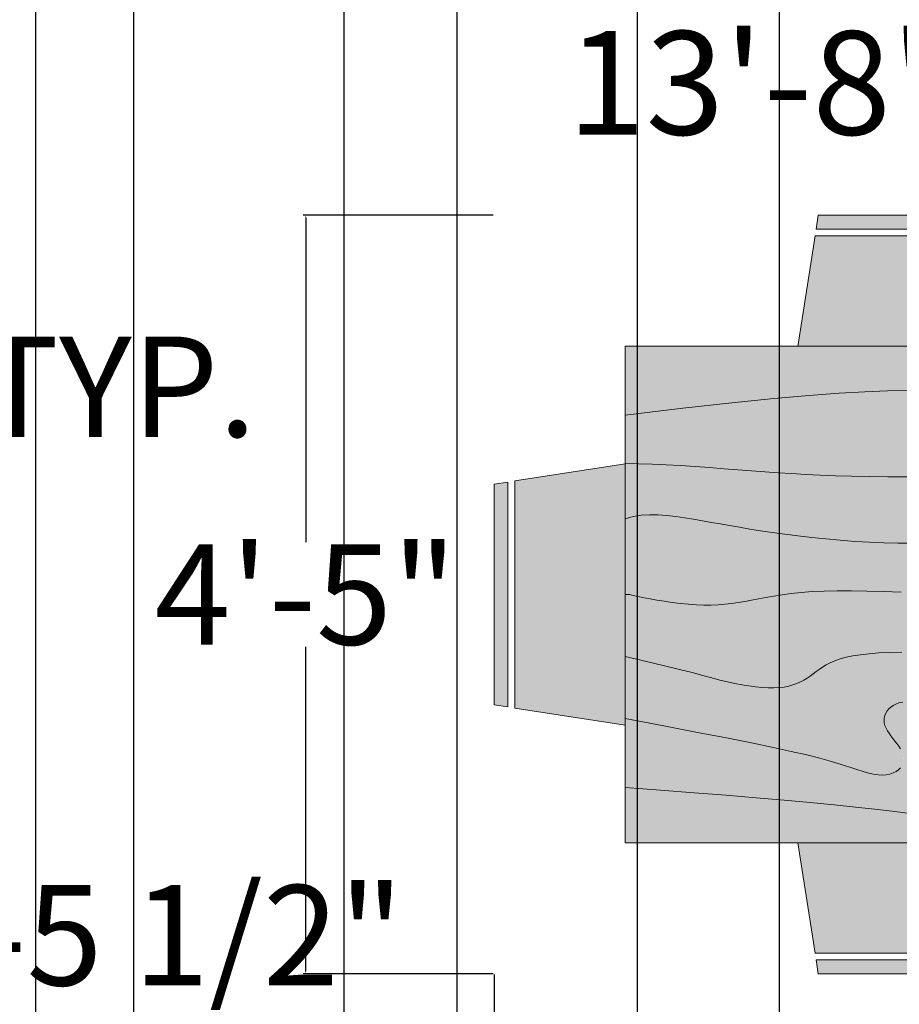
# Model space of a CAD drawing. Units: inches. Extents: x 2974 to 3443, y 2405 to 2963.
# Tile 5 of 13: x 3214 to 3276, y 2642 to 2711. Entities that reach past the tile are written whole.
import ezdxf

# ---------------------------------------------------------------- set-up
doc = ezdxf.new("R2010")
doc.units = ezdxf.units.IN
doc.header["$MEASUREMENT"] = 0
doc.layers.get('0').update_dxf_attribs({"color": 251})
for name, color, linetype, lineweight in [('A-ANNO-DIMS', 2, 'Continuous', 18), ('A-AREA-IDEN', 250, 'Continuous', 25), ('furniture', 32, 'Continuous', 18)]:
    doc.layers.add(name, color=color, linetype=linetype, lineweight=lineweight)
doc.layers.add('A-FURN-PATT', color=254, linetype='Continuous', lineweight=13, true_color=0xfeeab9)
doc.styles.get("Standard").update_dxf_attribs({"font": 'arial.ttf'})
doc.dimstyles.get("Standard").update_dxf_attribs({"dimtxt": 7, "dimasz": 0.18, "dimexe": 0.18, "dimexo": 0.0625, "dimgap": 0.09, "dimtad": 0, "dimtih": 1, "dimtoh": 1, "dimzin": 0, "dimdsep": 46, "dimlunit": 3, "dimtxsty": 'Standard', "dimcen": 0.09, "dimadec": 0, "dimazin": 0, "dimtfac": 1, "dimtofl": 0, "dimtmove": 0, "dimatfit": 3, "dimfxl": 1, "dimtolj": 1, "dimtzin": 0, "dimarcsym": 0})

# ---------------------------------------------------------------- blocks, each defined once
blk = doc.blocks.new('Dining Set - 36 x 72 in.')
for p, q in [((6, 27.5), (22, 27.5)), ((22.1563, 26.49966), (22, 27.5)), ((22.1584, 26.5), (5.8466, 26.5)), ((5.7696, 26), (22.2392, 26)), ((23.4848, 17.99762), (22.2345, 25.99926)), ((36, 18), (-36, 18)), ((36, -18), (36, 18)), ((44.0006, 8.23428), (35.9976, 9.48474)), ((44, 8.23041), (44, -8.23915)), ((44.5, -8.15843), (44.5, 8.15338)), ((45.5, 8), (44.5005, 8.15617)), ((45.5, 8), (45.5, -8)), ((35.9976, -9.48476), (43.9993, -8.2345)), ((44.4997, -8.15631), (45.5, -8)), ((-36, -18), (36, -18)), ((23.4848, -17.99762), (22.2345, -25.99928)), ((5.7696, -26), (22.2392, -26)), ((22.1584, -26.5), (5.8466, -26.5)), ((22.1563, -26.49967), (22, -27.5)), ((6, -27.5), (22, -27.5))]:
    blk.add_line(p, q)
for points in [[(15.5395, 15.84586), (16.6426, 15.71224), (17.8893, 15.56884), (19.2917, 15.41666), (20.859, 15.25667), (22.5879, 15.08984), (24.4721, 14.91715), (26.5052, 14.73958), (28.6809, 14.5581), (30.9929, 14.3737), (33.4347, 14.18733), (36, 14)], [(15.875, 7.80208), (16.1494, 7.86637), (16.3828, 7.94922), (16.5811, 8.04964), (16.75, 8.16666), (16.8944, 8.29915), (17.0143, 8.44531), (17.1089, 8.60319), (17.1771, 8.77083), (17.218, 8.94629), (17.2305, 9.1276), (17.2137, 9.31282), (17.1667, 9.5), (17.0895, 9.6875), (16.987, 9.875), (16.8649, 10.0625), (16.7292, 10.25), (16.5856, 10.4375), (16.4401, 10.625), (16.2985, 10.8125), (16.1667, 11), (16.05, 11.18733)], [(16.0295, 12.56836), (16.1784, 12.70833), (16.3605, 12.83268), (16.5729, 12.9375), (16.8127, 13.01888), (17.0768, 13.07291), (17.3625, 13.0957), (17.6667, 13.08333), (17.9894, 13.03312), (18.3418, 12.94726), (18.7382, 12.82918), (19.1927, 12.68229), (19.7195, 12.51001), (20.3327, 12.31575), (21.0465, 12.10294), (21.875, 11.875), (22.8357, 11.63354), (23.959, 11.37304), (25.2786, 11.08618), (26.8282, 10.76562), (28.6414, 10.40405), (30.752, 9.99414), (33.1936, 9.52856), (36, 9)], [(15.954, 4.17448), (16.819, 4.19791), (17.6001, 4.23698), (18.3021, 4.29166), (18.9299, 4.36198), (19.4883, 4.44791), (19.9823, 4.54948), (20.4167, 4.66666), (20.7969, 4.79899), (21.1302, 4.94401), (21.4245, 5.09879), (21.6875, 5.26041), (21.9271, 5.42594), (22.1511, 5.59245), (22.3672, 5.757), (22.5834, 5.91666), (22.8065, 6.06868), (23.0404, 6.21093), (23.2879, 6.34147), (23.5521, 6.45833), (23.8358, 6.55957), (24.142, 6.64323), (24.4735, 6.70735), (24.8334, 6.75), (25.2235, 6.76969), (25.642, 6.76692), (26.0858, 6.74267), (26.5521, 6.69791), (27.0379, 6.63362), (27.5404, 6.55078), (28.0565, 6.45036), (28.5834, 6.33333), (29.1242, 6.19987), (29.7071, 6.04687), (30.3661, 5.87044), (31.1354, 5.66666), (32.0493, 5.43164), (33.142, 5.16146), (34.4475, 4.85221), (36, 4.5)], [(15.9982, -0.17432), (17.2813, -0.21875), (18.4823, -0.25147), (19.6003, -0.26953), (20.6343, -0.27002), (21.5834, -0.25), (22.4481, -0.20768), (23.2357, -0.14584), (23.9549, -0.06836), (24.6146, 0.02083), (25.2235, 0.11784), (25.7904, 0.21875), (26.3241, 0.31966), (26.8334, 0.41666), (27.3265, 0.50618), (27.8099, 0.58593), (28.2894, 0.65397), (28.7709, 0.70833), (29.2601, 0.74707), (29.763, 0.76823), (30.2855, 0.76985), (30.8334, 0.75), (31.4088, 0.70784), (31.9994, 0.64713), (32.589, 0.57275), (33.1615, 0.48958), (33.7008, 0.4025), (34.1908, 0.3164), (34.6153, 0.23616), (34.9584, 0.16666), (35.2099, 0.11165), (35.3848, 0.07031), (35.504, 0.04069), (35.5886, 0.02083), (35.6594, 0.00879), (35.7377, 0.0026), (35.8442, 0.00032), (36, 0)], [(15.2266, -3.73177), (16.2295, -3.73015), (17.25, -3.75), (18.2912, -3.79248), (19.3451, -3.85547), (20.4009, -3.93604), (21.4479, -4.03125), (22.4754, -4.13819), (23.4727, -4.25391), (24.4289, -4.37549), (25.3334, -4.5), (26.1785, -4.62492), (26.9694, -4.74935), (27.7145, -4.87281), (28.4219, -4.99479), (29.1, -5.11483), (29.7572, -5.23242), (30.4016, -5.34709), (31.0417, -5.45834), (31.6837, -5.56437), (32.3262, -5.65821), (32.9658, -5.73153), (33.599, -5.77604), (34.2224, -5.78345), (34.8327, -5.74545), (35.4264, -5.65373), (36, -5.5)], [(15.4876, -8.53353), (16.9583, -8.53907), (18.3197, -8.55632), (19.5834, -8.58334), (20.7616, -8.61841), (21.8685, -8.66081), (22.9188, -8.71004), (23.9271, -8.76563), (24.9081, -8.82707), (25.8763, -8.89388), (26.8465, -8.96558), (27.8334, -9.04167), (28.8474, -9.12118), (29.8828, -9.20117), (30.93, -9.27824), (31.9792, -9.34896), (33.0205, -9.40991), (34.0443, -9.45768), (35.0407, -9.48885), (36, -9.5)], [(15.5417, -14.79167), (16.9933, -14.76424), (18.6152, -14.70508), (20.4804, -14.60197), (22.6615, -14.44271), (25.2312, -14.21509), (28.2624, -13.9069), (31.8277, -13.50594), (36, -13)]]:
    blk.add_lwpolyline(points)
blk = doc.blocks.new('dining area')
at = {"layer": 'furniture', "xscale": 0.6659924291999282, "yscale": 0.6659924291999282, "zscale": 0.6659924291999282, "rotation": 90}
blk.add_blockref('Dining Set - 36 x 72 in.', (-0.439, 20.507), dxfattribs=at)
blk = doc.blocks.new('*D35')
at = {"layer": 'A-ANNO-DIMS', "color": 0, "lineweight": -2, "transparency": 16777216}
for p, q in [((3110.658, 2681.378), (3110.658, 2685.223)), ((3135.509, 2681.378), (3135.509, 2685.223)), ((3110.838, 2685.043), (3135.329, 2685.043)), ((3135.509, 2685.043), (3135.689, 2685.043))]:
    blk.add_line(p, q, dxfattribs=at)
at = {"layer": 'A-ANNO-DIMS', "color": 0, "transparency": 16777216}
for points in [[(3110.838, 2685.073), (3110.838, 2685.013), (3110.658, 2685.043)], [(3135.329, 2685.073), (3135.329, 2685.013), (3135.509, 2685.043)]]:
    blk.add_solid(points, dxfattribs=at)
at = {"layer": 'Defpoints', "color": 0, "transparency": 16777216}
for p in [(3135.509, 2685.043), (3110.658, 2681.315), (3135.509, 2681.315)]:
    blk.add_point(p, dxfattribs=at)
at = {"layer": 'A-ANNO-DIMS', "color": 0, "transparency": 16777216, "insert": (3184.753, 2685.043), "char_height": 7, "attachment_point": 5}
blk.add_mtext('\\A1;ARMCHAIR 2\'-1" TYP.', dxfattribs=at)
blk = doc.blocks.new('*D46')
at = {"layer": 'A-ANNO-DIMS', "color": 0, "lineweight": -2, "transparency": 16777216}
for p, q in [((3199.048, 2640.453), (3199.048, 2646.942)), ((3199.228, 2646.762), (3204.43, 2646.762)), ((3204.61, 2640.453), (3204.61, 2646.942)), ((3204.61, 2646.762), (3204.79, 2646.762))]:
    blk.add_line(p, q, dxfattribs=at)
at = {"layer": 'A-ANNO-DIMS', "color": 0, "transparency": 16777216}
for points in [[(3199.228, 2646.792), (3199.228, 2646.732), (3199.048, 2646.762)], [(3204.43, 2646.792), (3204.43, 2646.732), (3204.61, 2646.762)]]:
    blk.add_solid(points, dxfattribs=at)
at = {"layer": 'Defpoints', "color": 0, "transparency": 16777216}
for p in [(3204.61, 2646.762), (3199.048, 2640.391), (3204.61, 2640.391)]:
    blk.add_point(p, dxfattribs=at)
at = {"layer": 'A-ANNO-DIMS', "color": 0, "transparency": 16777216, "insert": (3222.339, 2646.762), "char_height": 7, "attachment_point": 5}
blk.add_mtext('\\A1;0\'-5 1/2"', dxfattribs=at)
blk = doc.blocks.new('*D47')
at = {"layer": 'A-ANNO-DIMS', "color": 0, "lineweight": -2, "transparency": 16777216}
for p, q in [((3247.425, 2644.017), (3247.425, 2630.764)), ((3334.991, 2644.017), (3334.991, 2630.764)), ((3247.425, 2630.944), (3247.245, 2630.944)), ((3334.811, 2630.944), (3247.605, 2630.944))]:
    blk.add_line(p, q, dxfattribs=at)
at = {"layer": 'A-ANNO-DIMS', "color": 0, "transparency": 16777216}
for points in [[(3247.605, 2630.974), (3247.605, 2630.914), (3247.425, 2630.944)], [(3334.811, 2630.974), (3334.811, 2630.914), (3334.991, 2630.944)]]:
    blk.add_solid(points, dxfattribs=at)
at = {"layer": 'Defpoints', "color": 0, "transparency": 16777216}
for p in [(3247.425, 2644.079), (3334.991, 2644.079), (3247.425, 2630.944)]:
    blk.add_point(p, dxfattribs=at)
at = {"layer": 'A-ANNO-DIMS', "color": 0, "transparency": 16777216, "insert": (3200.531, 2630.944), "char_height": 7, "attachment_point": 5}
blk.add_mtext('\\A1;DINING SET 7\'-3 1/2"', dxfattribs=at)
blk = doc.blocks.new('*D48')
at = {"layer": 'A-ANNO-DIMS', "color": 0, "lineweight": -2, "transparency": 16777216}
for p, q in [((3247.363, 2697.003), (3234.11, 2697.003)), ((3234.29, 2696.823), (3234.29, 2674.191)), ((3234.29, 2644.259), (3234.29, 2666.892)), ((3247.363, 2644.079), (3234.11, 2644.079))]:
    blk.add_line(p, q, dxfattribs=at)
at = {"layer": 'A-ANNO-DIMS', "color": 0, "transparency": 16777216}
for points in [[(3234.26, 2696.823), (3234.32, 2696.823), (3234.29, 2697.003)], [(3234.26, 2644.259), (3234.32, 2644.259), (3234.29, 2644.079)]]:
    blk.add_solid(points, dxfattribs=at)
at = {"layer": 'Defpoints', "color": 0, "transparency": 16777216}
for p in [(3234.29, 2697.003), (3247.425, 2697.003), (3247.425, 2644.079)]:
    blk.add_point(p, dxfattribs=at)
at = {"layer": 'A-ANNO-DIMS', "color": 0, "transparency": 16777216, "insert": (3234.29, 2670.541), "char_height": 7, "attachment_point": 5}
blk.add_mtext('\\A1;4\'-5"', dxfattribs=at)
blk = doc.blocks.new('*D61')
at = {"layer": 'A-ANNO-DIMS', "color": 0, "lineweight": -2, "transparency": 16777216}
for p, q in [((3222.294, 2555.251), (3222.294, 2952.678)), ((3222.474, 2952.498), (3227.688, 2952.498)), ((3257.249, 2952.498), (3252.034, 2952.498)), ((3257.429, 2555.251), (3257.429, 2952.678))]:
    blk.add_line(p, q, dxfattribs=at)
at = {"layer": 'A-ANNO-DIMS', "color": 0, "transparency": 16777216}
for points in [[(3222.474, 2952.528), (3222.474, 2952.468), (3222.294, 2952.498)], [(3257.249, 2952.528), (3257.249, 2952.468), (3257.429, 2952.498)]]:
    blk.add_solid(points, dxfattribs=at)
at = {"layer": 'Defpoints', "color": 0, "transparency": 16777216}
for p in [(3257.429, 2952.498), (3222.294, 2555.188), (3257.429, 2555.188)]:
    blk.add_point(p, dxfattribs=at)
at = {"layer": 'A-ANNO-DIMS', "color": 0, "transparency": 16777216, "insert": (3239.861, 2952.498), "char_height": 7, "attachment_point": 5}
blk.add_mtext('\\A1;2\'-11"', dxfattribs=at)
blk = doc.blocks.new('*D62')
at = {"layer": 'A-ANNO-DIMS', "color": 0, "lineweight": -2, "transparency": 16777216}
for p, q in [((3267.326, 2609.251), (3267.326, 2952.678)), ((3267.506, 2952.498), (3281.115, 2952.498)), ((3329.823, 2952.498), (3316.214, 2952.498)), ((3330.003, 2609.251), (3330.003, 2952.678))]:
    blk.add_line(p, q, dxfattribs=at)
at = {"layer": 'A-ANNO-DIMS', "color": 0, "transparency": 16777216}
for points in [[(3267.506, 2952.528), (3267.506, 2952.468), (3267.326, 2952.498)], [(3329.823, 2952.528), (3329.823, 2952.468), (3330.003, 2952.498)]]:
    blk.add_solid(points, dxfattribs=at)
at = {"layer": 'Defpoints', "color": 0, "transparency": 16777216}
for p in [(3330.003, 2952.498), (3267.326, 2609.188), (3330.003, 2609.188)]:
    blk.add_point(p, dxfattribs=at)
at = {"layer": 'A-ANNO-DIMS', "color": 0, "transparency": 16777216, "insert": (3298.665, 2952.498), "char_height": 7, "attachment_point": 5}
blk.add_mtext('\\A1;5\'-2 1/2"', dxfattribs=at)
blk = doc.blocks.new('*D63')
at = {"layer": 'A-ANNO-DIMS', "color": 0, "lineweight": -2, "transparency": 16777216}
for p, q in [((3244.826, 2751.126), (3244.826, 2414.917)), ((3284.826, 2751.126), (3284.826, 2414.917)), ((3245.006, 2415.097), (3255.434, 2415.097)), ((3284.646, 2415.097), (3274.217, 2415.097))]:
    blk.add_line(p, q, dxfattribs=at)
at = {"layer": 'A-ANNO-DIMS', "color": 0, "transparency": 16777216}
for points in [[(3245.006, 2415.127), (3245.006, 2415.067), (3244.826, 2415.097)], [(3284.646, 2415.127), (3284.646, 2415.067), (3284.826, 2415.097)]]:
    blk.add_solid(points, dxfattribs=at)
at = {"layer": 'Defpoints', "color": 0, "transparency": 16777216}
for p in [(3244.826, 2751.188), (3284.826, 2751.188), (3284.826, 2415.097)]:
    blk.add_point(p, dxfattribs=at)
at = {"layer": 'A-ANNO-DIMS', "color": 0, "transparency": 16777216, "insert": (3264.826, 2415.097), "char_height": 7, "attachment_point": 5}
blk.add_mtext('\\A1;3\'-4"', dxfattribs=at)
blk = doc.blocks.new('*D65')
at = {"layer": 'A-ANNO-DIMS', "color": 0, "lineweight": -2, "transparency": 16777216}
for p, q in [((3215.45, 2808.126), (3215.45, 2414.917)), ((3236.952, 2808.126), (3236.952, 2414.917)), ((3215.63, 2415.097), (3236.772, 2415.097)), ((3236.952, 2415.097), (3237.132, 2415.097))]:
    blk.add_line(p, q, dxfattribs=at)
at = {"layer": 'A-ANNO-DIMS', "color": 0, "transparency": 16777216}
for points in [[(3215.63, 2415.127), (3215.63, 2415.067), (3215.45, 2415.097)], [(3236.772, 2415.127), (3236.772, 2415.067), (3236.952, 2415.097)]]:
    blk.add_solid(points, dxfattribs=at)
at = {"layer": 'Defpoints', "color": 0, "transparency": 16777216}
for p in [(3215.45, 2808.188), (3236.952, 2808.188), (3236.952, 2415.097)]:
    blk.add_point(p, dxfattribs=at)
at = {"layer": 'A-ANNO-DIMS', "color": 0, "transparency": 16777216, "insert": (3254.352, 2415.097), "char_height": 7, "attachment_point": 5}
blk.add_mtext('\\A1;1\'-9 1/2"', dxfattribs=at)
blk = doc.blocks.new('*D78')
at = {"layer": 'A-ANNO-DIMS', "color": 0, "lineweight": -2, "transparency": 16777216}
for p, q in [((3267.326, 2480.251), (3267.326, 2952.678)), ((3267.506, 2952.498), (3271.548, 2952.498)), ((3310.684, 2952.498), (3306.642, 2952.498)), ((3310.864, 2481.932), (3310.864, 2952.678))]:
    blk.add_line(p, q, dxfattribs=at)
at = {"layer": 'A-ANNO-DIMS', "color": 0, "transparency": 16777216}
for points in [[(3267.506, 2952.528), (3267.506, 2952.468), (3267.326, 2952.498)], [(3310.684, 2952.528), (3310.684, 2952.468), (3310.864, 2952.498)]]:
    blk.add_solid(points, dxfattribs=at)
at = {"layer": 'Defpoints', "color": 0, "transparency": 16777216}
for p in [(3310.864, 2952.498), (3310.864, 2481.869), (3267.326, 2480.188)]:
    blk.add_point(p, dxfattribs=at)
at = {"layer": 'A-ANNO-DIMS', "color": 0, "transparency": 16777216, "insert": (3289.095, 2952.498), "char_height": 7, "attachment_point": 5}
blk.add_mtext('\\A1;3\'-7 1/2"', dxfattribs=at)

msp = doc.modelspace()

# ---------------------------------------------------------------- hatches: boundary and pattern name
at = {"layer": 'A-FURN-PATT'}
h = msp.add_hatch(color=256, dxfattribs=at)
h.dxf.hatch_style = 1
h.paths.add_polyline_path([(3285.66, 2695.56), (3269.813, 2695.56), (3268.61, 2687.862), (3286.863, 2687.862)])
h.paths.add_polyline_path([(3285.434, 2697.003), (3270.038, 2697.003), (3269.888, 2696.041), (3285.585, 2696.041)])
h.paths.add_polyline_path([(3312.603, 2695.56), (3296.756, 2695.56), (3295.553, 2687.862), (3313.806, 2687.862)])
h.paths.add_polyline_path([(3312.378, 2697.003), (3296.981, 2697.003), (3296.831, 2696.041), (3312.528, 2696.041)])
h.paths.add_polyline_path([(3256.566, 2679.668), (3248.868, 2678.465), (3248.868, 2662.618), (3256.566, 2661.415)])
h.paths.add_polyline_path([(3248.387, 2678.39), (3247.425, 2678.239), (3247.425, 2662.843), (3248.387, 2662.693)])
h.paths.add_polyline_path([(3286.863, 2653.221), (3268.61, 2653.221), (3269.813, 2645.522), (3285.66, 2645.522)])
h.paths.add_polyline_path([(3285.585, 2645.041), (3269.888, 2645.041), (3270.038, 2644.079), (3285.434, 2644.079)])
h.paths.add_polyline_path([(3312.528, 2645.041), (3296.831, 2645.041), (3296.981, 2644.079), (3312.378, 2644.079)])
h.paths.add_polyline_path([(3313.806, 2653.221), (3295.553, 2653.221), (3296.756, 2645.522), (3312.603, 2645.522)])
h.paths.add_polyline_path([(3333.547, 2678.465), (3325.849, 2679.668), (3325.849, 2661.415), (3333.547, 2662.618)])
h.paths.add_polyline_path([(3334.991, 2678.239), (3334.028, 2678.39), (3334.028, 2662.693), (3334.991, 2662.843)])
h = msp.add_hatch(color=256, dxfattribs=at)
h.dxf.hatch_style = 1
h.paths.add_polyline_path([(3325.849, 2687.862), (3256.566, 2687.862), (3256.566, 2683.051), (3260.581, 2683.537), (3264.012, 2683.923), (3266.929, 2684.22), (3269.402, 2684.439), (3271.5, 2684.592), (3273.295, 2684.691), (3274.856, 2684.748), (3276.253, 2684.775), (3277.547, 2684.781), (3278.767, 2684.77), (3279.931, 2684.746), (3281.059, 2684.71), (3282.17, 2684.664), (3283.284, 2684.611), (3284.419, 2684.554), (3285.595, 2684.494), (3286.829, 2684.434), (3288.131, 2684.375), (3289.51, 2684.318), (3290.972, 2684.263), (3292.527, 2684.213), (3294.182, 2684.167), (3295.944, 2684.127), (3297.823, 2684.093), (3299.842, 2684.068), (3302.084, 2684.054), (3304.651, 2684.058), (3307.641, 2684.083), (3311.157, 2684.135), (3315.296, 2684.217), (3320.16, 2684.335), (3325.849, 2684.494)])
h.paths.add_polyline_path([(3325.849, 2684.494), (3320.16, 2684.335), (3315.296, 2684.217), (3311.157, 2684.135), (3307.641, 2684.083), (3304.651, 2684.058), (3302.084, 2684.054), (3299.842, 2684.068), (3297.823, 2684.093), (3295.944, 2684.127), (3294.182, 2684.167), (3292.527, 2684.213), (3290.972, 2684.263), (3289.51, 2684.318), (3288.131, 2684.375), (3286.829, 2684.434), (3285.595, 2684.494), (3284.419, 2684.554), (3283.284, 2684.611), (3282.17, 2684.664), (3281.059, 2684.71), (3279.931, 2684.746), (3278.767, 2684.77), (3277.547, 2684.781), (3276.253, 2684.775), (3274.856, 2684.748), (3273.295, 2684.691), (3271.5, 2684.592), (3269.402, 2684.439), (3266.929, 2684.22), (3264.012, 2683.923), (3260.581, 2683.537), (3256.566, 2683.051), (3256.566, 2679.683), (3257.49, 2679.672), (3258.448, 2679.642), (3259.434, 2679.596), (3260.436, 2679.537), (3261.445, 2679.469), (3262.453, 2679.395), (3263.449, 2679.318), (3264.425, 2679.242), (3265.375, 2679.168), (3266.308, 2679.099), (3267.24, 2679.035), (3268.184, 2678.976), (3269.154, 2678.923), (3270.165, 2678.875), (3271.23, 2678.834), (3272.364, 2678.801), (3273.58, 2678.775), (3274.89, 2678.758), (3276.305, 2678.753), (3277.836, 2678.761), (3279.496, 2678.783), (3281.295, 2678.823), (3283.244, 2678.882), (3285.354, 2678.961), (3287.67, 2679.062), (3290.362, 2679.183), (3293.635, 2679.32), (3297.693, 2679.472), (3302.739, 2679.635), (3308.978, 2679.807), (3316.614, 2679.984), (3325.849, 2680.164)])
h.paths.add_polyline_path([(3284.707, 2677.646), (3284.542, 2678.931), (3283.244, 2678.882), (3281.295, 2678.823), (3279.496, 2678.783), (3277.836, 2678.761), (3276.305, 2678.753), (3274.89, 2678.758), (3273.58, 2678.775), (3272.364, 2678.801), (3271.23, 2678.834), (3270.165, 2678.875), (3269.154, 2678.923), (3268.184, 2678.976), (3267.24, 2679.035), (3266.308, 2679.099), (3265.375, 2679.168), (3264.425, 2679.242), (3263.449, 2679.318), (3262.453, 2679.395), (3261.445, 2679.469), (3260.436, 2679.537), (3259.434, 2679.596), (3258.448, 2679.642), (3257.49, 2679.672), (3256.656, 2679.682), (3256.566, 2679.668), (3256.566, 2675.834), (3257.118, 2675.982), (3257.69, 2676.07), (3258.277, 2676.106), (3258.877, 2676.099), (3259.486, 2676.056), (3260.102, 2675.986), (3260.72, 2675.896), (3261.338, 2675.794), (3261.954, 2675.687), (3262.574, 2675.576), (3263.206, 2675.463), (3263.859, 2675.348), (3264.539, 2675.23), (3265.256, 2675.111), (3266.017, 2674.992), (3266.831, 2674.871), (3267.701, 2674.752), (3268.621, 2674.635), (3269.581, 2674.523), (3270.569, 2674.42), (3271.577, 2674.329), (3272.593, 2674.251), (3273.607, 2674.191), (3274.609, 2674.15), (3275.591, 2674.131), (3276.556, 2674.132), (3277.51, 2674.153), (3278.458, 2674.19), (3279.406, 2674.242), (3280.36, 2674.308), (3281.325, 2674.384), (3282.307, 2674.47), (3283.312, 2674.564), (3284.35, 2674.666), (3285.43, 2674.775), (3286.562, 2674.891), (3287.756, 2675.015), (3288.049, 2675.046)])
h.paths.add_polyline_path([(3288.532, 2674.053), (3285.273, 2674.759), (3284.35, 2674.666), (3283.312, 2674.564), (3282.307, 2674.47), (3281.325, 2674.384), (3280.36, 2674.308), (3279.406, 2674.242), (3278.458, 2674.19), (3277.51, 2674.153), (3276.556, 2674.132), (3275.591, 2674.131), (3274.609, 2674.15), (3273.607, 2674.191), (3272.593, 2674.251), (3271.577, 2674.329), (3270.569, 2674.42), (3269.581, 2674.523), (3268.621, 2674.635), (3267.701, 2674.752), (3266.831, 2674.871), (3266.017, 2674.992), (3265.256, 2675.111), (3264.539, 2675.23), (3263.859, 2675.348), (3263.206, 2675.463), (3262.574, 2675.576), (3261.954, 2675.687), (3261.338, 2675.794), (3260.72, 2675.896), (3260.102, 2675.986), (3259.486, 2676.056), (3258.877, 2676.099), (3258.277, 2676.106), (3257.69, 2676.07), (3257.118, 2675.982), (3256.566, 2675.834), (3256.566, 2670.541), (3256.88, 2670.541), (3257.044, 2670.502), (3257.158, 2670.474), (3257.327, 2670.434), (3257.569, 2670.381), (3257.899, 2670.314), (3258.307, 2670.237), (3258.779, 2670.154), (3259.298, 2670.07), (3259.849, 2669.99), (3260.416, 2669.919), (3260.984, 2669.86), (3261.538, 2669.82), (3262.065, 2669.8), (3262.568, 2669.802), (3263.052, 2669.822), (3263.523, 2669.86), (3263.986, 2669.912), (3264.447, 2669.977), (3264.913, 2670.054), (3265.387, 2670.14), (3265.877, 2670.234), (3266.391, 2670.331), (3266.936, 2670.428), (3267.522, 2670.521), (3268.157, 2670.607), (3268.849, 2670.682), (3269.607, 2670.741), (3270.439, 2670.782), (3271.352, 2670.801), (3272.347, 2670.801), (3273.423, 2670.783), (3274.579, 2670.752), (3275.813, 2670.709), (3277.126, 2670.658), (3278.516, 2670.601), (3279.981, 2670.541), (3281.525, 2670.481), (3283.16, 2670.424), (3284.902, 2670.371), (3286.767, 2670.326), (3288.772, 2670.289), (3289.667, 2670.279), (3289.783, 2670.301)], flags=16)
h.paths.add_polyline_path([(3325.849, 2680.164), (3316.614, 2679.984), (3308.978, 2679.807), (3302.739, 2679.635), (3297.693, 2679.472), (3293.635, 2679.32), (3290.362, 2679.183), (3287.67, 2679.062), (3285.354, 2678.961), (3284.542, 2678.931), (3284.707, 2677.646), (3288.049, 2675.046), (3289.022, 2675.147), (3290.37, 2675.286), (3291.809, 2675.433), (3293.55, 2675.603), (3293.55, 2675.601), (3295.284, 2675.747), (3297.727, 2675.913), (3300.936, 2676.084), (3305.131, 2676.259), (3310.534, 2676.436), (3317.366, 2676.616), (3325.849, 2676.796)])
h.paths.add_polyline_path([(3325.849, 2676.796), (3317.366, 2676.616), (3310.534, 2676.436), (3305.131, 2676.259), (3300.936, 2676.084), (3297.727, 2675.913), (3297.25, 2675.881), (3296.279, 2674.149), (3296.261, 2674.155), (3293.605, 2673.358), (3290.309, 2670.721), (3292.302, 2670.259), (3293.261, 2670.255), (3295.779, 2670.261), (3298.501, 2670.286), (3301.458, 2670.336), (3304.68, 2670.418), (3308.198, 2670.536), (3312.043, 2670.698), (3316.245, 2670.909), (3320.837, 2671.175), (3325.849, 2671.503)])
h.paths.add_polyline_path([(3325.849, 2671.503), (3320.837, 2671.175), (3316.245, 2670.909), (3312.043, 2670.698), (3308.198, 2670.536), (3304.68, 2670.418), (3301.458, 2670.336), (3298.501, 2670.286), (3295.779, 2670.261), (3293.261, 2670.255), (3290.931, 2670.265), (3289.803, 2670.278), (3292.302, 2667.394), (3292.338, 2667.4), (3292.346, 2667.343), (3293.095, 2666.479), (3294.056, 2665.913), (3295.113, 2665.884), (3296.894, 2665.844), (3298.826, 2665.81), (3300.937, 2665.783), (3303.285, 2665.756), (3305.931, 2665.724), (3308.94, 2665.68), (3312.372, 2665.617), (3316.293, 2665.528), (3320.764, 2665.408), (3325.849, 2665.249)])
h.paths.add_polyline_path([(3325.849, 2665.249), (3320.764, 2665.408), (3316.293, 2665.528), (3312.372, 2665.617), (3308.94, 2665.68), (3305.931, 2665.724), (3303.285, 2665.756), (3300.937, 2665.783), (3298.826, 2665.81), (3296.894, 2665.844), (3295.113, 2665.884), (3294.056, 2665.913), (3293.095, 2666.479), (3292.346, 2667.343), (3289.803, 2670.278), (3289.78, 2670.278), (3289.019, 2664.95), (3288.717, 2664.649), (3288.853, 2661.906), (3289.258, 2661.871), (3290.783, 2661.741), (3292.386, 2661.607), (3294.066, 2661.466), (3295.819, 2661.32), (3297.67, 2661.168), (3299.75, 2661.02), (3302.216, 2660.89), (3305.226, 2660.788), (3308.937, 2660.728), (3313.506, 2660.722), (3319.091, 2660.781), (3325.849, 2660.919)])
h.paths.add_polyline_path([(3289.431, 2667.834), (3289.783, 2670.301), (3288.532, 2674.053), (3285.273, 2674.759), (3284.35, 2674.666), (3283.312, 2674.564), (3282.307, 2674.47), (3281.325, 2674.384), (3280.36, 2674.308), (3279.406, 2674.242), (3278.458, 2674.19), (3277.51, 2674.153), (3276.556, 2674.132), (3275.591, 2674.131), (3274.609, 2674.15), (3273.607, 2674.191), (3272.593, 2674.251), (3271.577, 2674.329), (3270.569, 2674.42), (3269.581, 2674.523), (3268.621, 2674.635), (3267.701, 2674.752), (3266.831, 2674.871), (3266.017, 2674.992), (3265.256, 2675.111), (3264.539, 2675.23), (3263.859, 2675.348), (3263.206, 2675.463), (3262.574, 2675.576), (3261.954, 2675.687), (3261.338, 2675.794), (3260.72, 2675.896), (3260.102, 2675.986), (3259.486, 2676.056), (3258.877, 2676.099), (3258.277, 2676.106), (3257.69, 2676.07), (3257.118, 2675.982), (3256.566, 2675.834), (3256.566, 2670.541), (3256.88, 2670.541), (3257.044, 2670.502), (3257.158, 2670.474), (3257.442, 2670.406), (3257.569, 2670.381), (3257.258, 2670.449), (3257.044, 2670.502), (3256.88, 2670.541), (3256.566, 2670.541), (3256.566, 2666.211), (3258.06, 2665.872), (3259.317, 2665.575), (3260.368, 2665.315), (3261.247, 2665.088), (3261.988, 2664.892), (3262.622, 2664.723), (3263.183, 2664.575), (3263.703, 2664.447), (3264.21, 2664.334), (3264.707, 2664.238), (3265.19, 2664.158), (3265.658, 2664.096), (3266.107, 2664.053), (3266.534, 2664.03), (3266.936, 2664.027), (3267.312, 2664.046), (3267.658, 2664.087), (3267.977, 2664.149), (3268.272, 2664.229), (3268.545, 2664.327), (3268.799, 2664.439), (3269.037, 2664.565), (3269.262, 2664.702), (3269.477, 2664.848), (3269.685, 2665.002), (3270.053, 2665.282), (3270.339, 2665.479), (3270.592, 2665.635), (3270.875, 2665.784), (3271.196, 2665.923), (3271.562, 2666.051), (3271.98, 2666.163), (3272.455, 2666.261), (3272.992, 2666.344), (3273.596, 2666.412), (3274.272, 2666.464), (3275.024, 2666.502), (3275.856, 2666.524), (3276.774, 2666.532), (3277.779, 2666.525), (3278.864, 2666.504), (3280.016, 2666.473), (3281.224, 2666.432), (3282.478, 2666.383), (3283.765, 2666.329), (3285.075, 2666.271), (3286.397, 2666.211), (3287.075, 2666.18)])
h.paths.add_polyline_path([(3289.019, 2664.95), (3289.431, 2667.834), (3287.075, 2666.18), (3286.397, 2666.211), (3285.075, 2666.271), (3283.765, 2666.329), (3282.478, 2666.383), (3281.224, 2666.432), (3280.016, 2666.473), (3278.864, 2666.504), (3277.779, 2666.525), (3276.774, 2666.532), (3275.856, 2666.524), (3275.024, 2666.502), (3274.272, 2666.464), (3273.596, 2666.412), (3272.992, 2666.344), (3272.455, 2666.261), (3271.98, 2666.163), (3271.562, 2666.051), (3271.196, 2665.923), (3270.875, 2665.784), (3270.592, 2665.635), (3270.339, 2665.479), (3270.053, 2665.282), (3269.536, 2664.889), (3269.144, 2664.621), (3268.799, 2664.439), (3268.545, 2664.327), (3268.272, 2664.229), (3267.977, 2664.149), (3267.658, 2664.087), (3267.312, 2664.046), (3266.936, 2664.027), (3266.534, 2664.03), (3266.107, 2664.053), (3265.658, 2664.096), (3265.19, 2664.158), (3264.707, 2664.238), (3264.21, 2664.334), (3263.703, 2664.447), (3263.183, 2664.575), (3262.622, 2664.723), (3261.988, 2664.892), (3261.247, 2665.088), (3260.368, 2665.315), (3259.317, 2665.575), (3258.06, 2665.872), (3256.566, 2666.211), (3256.566, 2661.881), (3259.267, 2661.372), (3261.616, 2660.924), (3263.647, 2660.53), (3265.392, 2660.182), (3266.883, 2659.873), (3268.153, 2659.597), (3269.234, 2659.347), (3270.158, 2659.114), (3270.956, 2658.895), (3271.643, 2658.69), (3272.233, 2658.503), (3272.739, 2658.338), (3273.177, 2658.196), (3273.558, 2658.083), (3273.897, 2658), (3274.208, 2657.952), (3274.501, 2657.94), (3274.776, 2657.962), (3275.03, 2658.014), (3275.26, 2658.092), (3275.465, 2658.193), (3275.64, 2658.313), (3275.783, 2658.447), (3275.892, 2658.593), (3275.964, 2658.747), (3276.001, 2658.908), (3276.006, 2659.074), (3275.982, 2659.245), (3275.932, 2659.419), (3275.858, 2659.597), (3275.764, 2659.776), (3275.651, 2659.956), (3275.524, 2660.137), (3275.388, 2660.317), (3275.135, 2660.643), (3274.902, 2660.965), (3274.71, 2661.317), (3274.621, 2661.669), (3274.646, 2662.019), (3274.778, 2662.344), (3275.01, 2662.628), (3275.338, 2662.855), (3275.668, 2662.972), (3275.932, 2663.034), (3276.241, 2663.077), (3276.601, 2663.1), (3277.017, 2663.103), (3277.496, 2663.084), (3278.041, 2663.043), (3278.657, 2662.982), (3279.346, 2662.905), (3280.112, 2662.813), (3280.956, 2662.71), (3281.882, 2662.599), (3282.893, 2662.482), (3283.991, 2662.362), (3285.178, 2662.242), (3286.212, 2662.143)])
h.paths.add_polyline_path([(3288.532, 2674.053), (3285.273, 2674.759), (3284.35, 2674.666), (3283.312, 2674.564), (3282.307, 2674.47), (3281.325, 2674.384), (3280.36, 2674.308), (3279.406, 2674.242), (3278.458, 2674.19), (3277.51, 2674.153), (3276.556, 2674.132), (3275.591, 2674.131), (3274.609, 2674.15), (3273.607, 2674.191), (3272.593, 2674.251), (3271.577, 2674.329), (3270.569, 2674.42), (3269.581, 2674.523), (3268.621, 2674.635), (3267.701, 2674.752), (3266.831, 2674.871), (3266.017, 2674.992), (3265.256, 2675.111), (3264.539, 2675.23), (3263.859, 2675.348), (3263.206, 2675.463), (3262.574, 2675.576), (3261.954, 2675.687), (3261.338, 2675.794), (3260.72, 2675.896), (3260.102, 2675.986), (3259.486, 2676.056), (3258.877, 2676.099), (3258.277, 2676.106), (3257.69, 2676.07), (3257.118, 2675.982), (3256.566, 2675.834), (3256.566, 2670.541), (3256.716, 2670.541), (3256.88, 2670.541), (3257.044, 2670.502), (3257.158, 2670.474), (3257.327, 2670.434), (3257.569, 2670.381), (3257.899, 2670.314), (3258.307, 2670.237), (3258.779, 2670.154), (3259.298, 2670.07), (3259.849, 2669.99), (3260.416, 2669.919), (3260.984, 2669.86), (3261.538, 2669.82), (3262.065, 2669.8), (3262.568, 2669.802), (3263.052, 2669.822), (3263.523, 2669.86), (3263.986, 2669.912), (3264.447, 2669.977), (3264.913, 2670.054), (3265.387, 2670.14), (3265.877, 2670.234), (3266.391, 2670.331), (3266.936, 2670.428), (3267.522, 2670.521), (3268.157, 2670.607), (3268.849, 2670.682), (3269.607, 2670.741), (3270.439, 2670.782), (3271.352, 2670.801), (3272.347, 2670.801), (3273.423, 2670.783), (3274.579, 2670.752), (3275.813, 2670.709), (3277.126, 2670.658), (3278.516, 2670.601), (3279.981, 2670.541), (3281.525, 2670.481), (3283.16, 2670.424), (3284.902, 2670.371), (3286.767, 2670.326), (3288.772, 2670.289), (3289.667, 2670.279), (3289.783, 2670.301)], flags=17)
h.paths.add_polyline_path([(3275.26, 2658.092), (3275.465, 2658.193), (3275.64, 2658.313), (3275.783, 2658.447), (3275.892, 2658.593), (3275.964, 2658.747), (3276.001, 2658.908), (3276.006, 2659.074), (3275.982, 2659.245), (3275.932, 2659.419), (3275.858, 2659.597), (3275.764, 2659.776), (3275.651, 2659.956), (3275.524, 2660.137), (3275.388, 2660.317), (3275.038, 2660.768), (3274.979, 2660.858), (3274.902, 2660.965), (3274.71, 2661.317), (3274.621, 2661.669), (3274.646, 2662.019), (3274.778, 2662.344), (3275.01, 2662.628), (3275.338, 2662.855), (3275.668, 2662.972), (3275.932, 2663.034), (3276.241, 2663.077), (3276.601, 2663.1), (3277.017, 2663.103), (3277.496, 2663.084), (3278.041, 2663.043), (3278.657, 2662.982), (3279.346, 2662.905), (3280.112, 2662.813), (3280.956, 2662.71), (3281.882, 2662.599), (3282.893, 2662.482), (3283.991, 2662.362), (3285.178, 2662.242), (3286.212, 2662.143), (3289.019, 2664.95), (3289.431, 2667.834), (3287.075, 2666.18), (3286.397, 2666.211), (3285.075, 2666.271), (3283.765, 2666.329), (3282.478, 2666.383), (3281.224, 2666.432), (3280.016, 2666.473), (3278.864, 2666.504), (3277.779, 2666.525), (3276.774, 2666.532), (3275.856, 2666.524), (3275.024, 2666.502), (3274.272, 2666.464), (3273.596, 2666.412), (3272.992, 2666.344), (3272.455, 2666.261), (3271.98, 2666.163), (3271.562, 2666.051), (3271.196, 2665.923), (3270.875, 2665.784), (3270.592, 2665.635), (3270.339, 2665.479), (3270.053, 2665.282), (3269.536, 2664.889), (3269.144, 2664.621), (3268.799, 2664.439), (3268.545, 2664.327), (3268.272, 2664.229), (3267.977, 2664.149), (3267.658, 2664.087), (3267.312, 2664.046), (3266.936, 2664.027), (3266.534, 2664.03), (3266.107, 2664.053), (3265.658, 2664.096), (3265.19, 2664.158), (3264.707, 2664.238), (3264.21, 2664.334), (3263.703, 2664.447), (3263.183, 2664.575), (3262.622, 2664.723), (3261.988, 2664.892), (3261.247, 2665.088), (3260.368, 2665.315), (3259.317, 2665.575), (3258.06, 2665.872), (3256.566, 2666.211), (3256.566, 2661.881), (3259.267, 2661.372), (3261.616, 2660.924), (3263.647, 2660.53), (3265.392, 2660.182), (3266.883, 2659.873), (3268.153, 2659.597), (3269.234, 2659.347), (3270.158, 2659.114), (3270.956, 2658.895), (3271.643, 2658.69), (3272.233, 2658.503), (3272.739, 2658.338), (3273.177, 2658.196), (3273.558, 2658.083), (3273.897, 2658), (3274.208, 2657.952), (3274.501, 2657.94), (3274.776, 2657.962), (3275.03, 2658.014)], flags=16)
h.paths.add_polyline_path([(3286.212, 2662.143), (3285.178, 2662.242), (3283.991, 2662.362), (3282.893, 2662.482), (3281.882, 2662.599), (3280.956, 2662.71), (3280.112, 2662.813), (3279.346, 2662.905), (3278.657, 2662.982), (3278.041, 2663.043), (3277.496, 2663.084), (3277.017, 2663.103), (3276.601, 2663.1), (3276.241, 2663.077), (3275.932, 2663.034), (3275.668, 2662.972), (3275.443, 2662.892), (3275.253, 2662.795), (3275.09, 2662.683), (3274.951, 2662.555), (3274.836, 2662.415), (3274.745, 2662.263), (3274.679, 2662.101), (3274.64, 2661.933), (3274.628, 2661.758), (3274.644, 2661.58), (3274.689, 2661.4), (3274.763, 2661.219), (3274.862, 2661.039), (3274.979, 2660.858), (3275.11, 2660.678), (3275.248, 2660.498), (3275.488, 2660.188), (3275.72, 2659.858), (3275.908, 2659.502), (3276.009, 2659.153), (3275.998, 2658.821), (3275.855, 2658.515), (3275.566, 2658.243), (3275.153, 2658.039), (3274.776, 2657.962), (3274.501, 2657.94), (3274.208, 2657.952), (3273.897, 2658), (3273.558, 2658.083), (3273.177, 2658.196), (3272.739, 2658.338), (3272.233, 2658.503), (3271.643, 2658.69), (3270.956, 2658.895), (3270.158, 2659.114), (3269.234, 2659.347), (3268.153, 2659.597), (3266.883, 2659.873), (3265.392, 2660.182), (3263.647, 2660.53), (3261.616, 2660.924), (3259.267, 2661.372), (3256.566, 2661.881), (3256.566, 2657.07), (3259.035, 2656.889), (3261.385, 2656.71), (3263.609, 2656.533), (3265.703, 2656.358), (3267.659, 2656.187), (3269.472, 2656.021), (3271.136, 2655.86), (3272.644, 2655.706), (3273.994, 2655.56), (3275.193, 2655.422), (3276.255, 2655.293), (3277.19, 2655.175), (3278.01, 2655.068), (3278.728, 2654.973), (3279.354, 2654.892), (3279.901, 2654.824), (3280.38, 2654.772), (3280.796, 2654.734), (3281.156, 2654.712), (3281.465, 2654.704), (3281.729, 2654.712), (3281.954, 2654.734), (3282.144, 2654.772), (3282.307, 2654.824), (3282.446, 2654.892), (3282.563, 2654.972), (3282.657, 2655.064), (3282.728, 2655.165), (3282.777, 2655.274), (3282.803, 2655.388), (3282.807, 2655.506), (3282.788, 2655.626), (3282.747, 2655.747), (3282.689, 2655.868), (3282.618, 2655.991), (3282.538, 2656.117), (3282.335, 2656.431), (3282.191, 2656.747), (3282.122, 2657.065), (3282.142, 2657.385), (3282.273, 2657.684), (3282.54, 2657.942), (3282.863, 2658.079), (3283.155, 2658.156), (3283.53, 2658.212), (3284.002, 2658.246), (3284.587, 2658.255), (3285.3, 2658.238), (3286.156, 2658.192), (3287.168, 2658.118), (3288.339, 2658.017), (3289.674, 2657.893), (3291.173, 2657.751), (3292.839, 2657.594), (3294.675, 2657.425), (3296.684, 2657.249), (3298.866, 2657.07), (3301.231, 2656.89), (3303.809, 2656.716), (3306.639, 2656.554), (3309.756, 2656.408), (3313.199, 2656.285), (3317.004, 2656.19), (3321.208, 2656.129), (3325.849, 2656.107), (3325.849, 2660.919), (3319.091, 2660.781), (3313.506, 2660.722), (3308.937, 2660.728), (3305.226, 2660.788), (3302.216, 2660.89), (3299.75, 2661.02), (3297.67, 2661.168), (3295.819, 2661.32), (3294.066, 2661.466), (3292.386, 2661.607), (3290.783, 2661.741), (3289.258, 2661.871), (3287.725, 2662.005), (3287.725, 2662.005), (3286.211, 2662.142)])
h.paths.add_polyline_path([(3289.019, 2664.95), (3289.431, 2667.834), (3287.075, 2666.18), (3286.397, 2666.211), (3285.075, 2666.271), (3283.765, 2666.329), (3282.478, 2666.383), (3281.224, 2666.432), (3280.016, 2666.473), (3278.864, 2666.504), (3277.779, 2666.525), (3276.774, 2666.532), (3275.856, 2666.524), (3275.024, 2666.502), (3274.272, 2666.464), (3273.596, 2666.412), (3272.992, 2666.344), (3272.455, 2666.261), (3271.98, 2666.163), (3271.562, 2666.051), (3271.196, 2665.923), (3270.875, 2665.784), (3270.592, 2665.635), (3270.339, 2665.479), (3270.053, 2665.282), (3269.536, 2664.889), (3269.144, 2664.621), (3268.799, 2664.439), (3268.545, 2664.327), (3268.272, 2664.229), (3267.977, 2664.149), (3267.658, 2664.087), (3267.312, 2664.046), (3266.936, 2664.027), (3266.534, 2664.03), (3266.107, 2664.053), (3265.658, 2664.096), (3265.19, 2664.158), (3264.707, 2664.238), (3264.21, 2664.334), (3263.703, 2664.447), (3263.183, 2664.575), (3262.622, 2664.723), (3261.988, 2664.892), (3261.247, 2665.088), (3260.368, 2665.315), (3259.317, 2665.575), (3258.06, 2665.872), (3256.566, 2666.211), (3256.566, 2661.881), (3259.267, 2661.372), (3261.616, 2660.924), (3263.647, 2660.53), (3265.392, 2660.182), (3266.883, 2659.873), (3268.153, 2659.597), (3269.234, 2659.347), (3270.158, 2659.114), (3270.956, 2658.895), (3271.643, 2658.69), (3272.233, 2658.503), (3272.739, 2658.338), (3273.177, 2658.196), (3273.558, 2658.083), (3273.897, 2658), (3274.208, 2657.952), (3274.501, 2657.94), (3274.776, 2657.962), (3275.03, 2658.014), (3275.26, 2658.092), (3275.465, 2658.193), (3275.64, 2658.313), (3275.783, 2658.447), (3275.892, 2658.593), (3275.964, 2658.747), (3276.001, 2658.908), (3276.006, 2659.074), (3275.982, 2659.245), (3275.932, 2659.419), (3275.858, 2659.597), (3275.764, 2659.776), (3275.651, 2659.956), (3275.524, 2660.137), (3275.388, 2660.317), (3275.248, 2660.498), (3274.942, 2660.892), (3274.71, 2661.317), (3274.644, 2661.58), (3274.621, 2661.669), (3274.64, 2661.933), (3274.646, 2662.019), (3274.745, 2662.263), (3274.778, 2662.344), (3274.951, 2662.555), (3275.01, 2662.628), (3275.253, 2662.795), (3275.338, 2662.855), (3275.668, 2662.972), (3275.932, 2663.034), (3276.241, 2663.077), (3276.601, 2663.1), (3277.017, 2663.103), (3277.496, 2663.084), (3278.041, 2663.043), (3278.657, 2662.982), (3279.346, 2662.905), (3280.112, 2662.813), (3280.956, 2662.71), (3281.882, 2662.599), (3282.893, 2662.482), (3283.991, 2662.362), (3285.178, 2662.242), (3286.212, 2662.143)], flags=17)
h.paths.add_polyline_path([(3286.397, 2666.211), (3285.075, 2666.271), (3283.765, 2666.329), (3282.478, 2666.383), (3281.224, 2666.432), (3280.016, 2666.473), (3278.864, 2666.504), (3277.779, 2666.525), (3276.774, 2666.532), (3275.856, 2666.524), (3275.024, 2666.502), (3274.272, 2666.464), (3273.596, 2666.412), (3272.992, 2666.344), (3272.455, 2666.261), (3271.98, 2666.163), (3271.562, 2666.051), (3271.196, 2665.923), (3270.875, 2665.784), (3270.592, 2665.635), (3270.339, 2665.479), (3270.108, 2665.32), (3269.893, 2665.16), (3269.685, 2665.002), (3269.536, 2664.889), (3269.144, 2664.621), (3268.799, 2664.439), (3268.545, 2664.327), (3268.272, 2664.229), (3267.977, 2664.149), (3267.658, 2664.087), (3267.312, 2664.046), (3266.936, 2664.027), (3266.534, 2664.03), (3266.107, 2664.053), (3265.658, 2664.096), (3265.19, 2664.158), (3264.707, 2664.238), (3264.21, 2664.334), (3263.703, 2664.447), (3263.183, 2664.575), (3262.622, 2664.723), (3261.988, 2664.892), (3261.247, 2665.088), (3260.368, 2665.315), (3259.317, 2665.575), (3258.06, 2665.872), (3256.566, 2666.211), (3256.566, 2661.881), (3259.267, 2661.372), (3261.616, 2660.924), (3263.647, 2660.53), (3265.392, 2660.182), (3266.883, 2659.873), (3268.153, 2659.597), (3269.234, 2659.347), (3270.158, 2659.114), (3270.956, 2658.895), (3271.643, 2658.69), (3272.233, 2658.503), (3272.739, 2658.338), (3273.177, 2658.196), (3273.558, 2658.083), (3273.897, 2658), (3274.208, 2657.952), (3274.501, 2657.94), (3274.776, 2657.962), (3275.03, 2658.014), (3275.26, 2658.092), (3275.465, 2658.193), (3275.64, 2658.313), (3275.783, 2658.447), (3275.892, 2658.593), (3275.964, 2658.747), (3276.001, 2658.908), (3276.006, 2659.074), (3275.982, 2659.245), (3275.932, 2659.419), (3275.858, 2659.597), (3275.764, 2659.776), (3275.651, 2659.956), (3275.524, 2660.137), (3275.388, 2660.317), (3275.248, 2660.498), (3274.942, 2660.892), (3274.71, 2661.317), (3274.644, 2661.58), (3274.621, 2661.669), (3274.64, 2661.933), (3274.646, 2662.019), (3274.745, 2662.263), (3274.778, 2662.344), (3274.951, 2662.555), (3275.01, 2662.628), (3275.253, 2662.795), (3275.338, 2662.855), (3275.668, 2662.972), (3275.932, 2663.034), (3276.241, 2663.077), (3276.601, 2663.1), (3277.017, 2663.103), (3277.496, 2663.084), (3278.041, 2663.043), (3278.657, 2662.982), (3279.346, 2662.905), (3280.112, 2662.813), (3280.956, 2662.71), (3281.882, 2662.599), (3282.893, 2662.482), (3283.991, 2662.362), (3285.178, 2662.242), (3286.212, 2662.143), (3289.019, 2664.95), (3289.181, 2666.088), (3289.072, 2666.092), (3287.723, 2666.151)], flags=0)
h.paths.add_polyline_path([(3288.717, 2664.649), (3287.458, 2663.39), (3287.725, 2662.005), (3287.814, 2661.997), (3288.853, 2661.906)], flags=0)
h.paths.add_polyline_path([(3287.458, 2663.39), (3286.212, 2662.143), (3286.454, 2662.12), (3287.725, 2662.005)], flags=0)
h.paths.add_polyline_path([(3325.849, 2656.107), (3321.208, 2656.129), (3317.004, 2656.19), (3313.199, 2656.285), (3309.756, 2656.408), (3306.639, 2656.554), (3303.809, 2656.716), (3301.231, 2656.89), (3298.866, 2657.07), (3296.684, 2657.249), (3294.675, 2657.425), (3292.839, 2657.594), (3291.173, 2657.751), (3289.674, 2657.893), (3288.339, 2658.017), (3287.168, 2658.118), (3286.156, 2658.192), (3285.3, 2658.238), (3284.587, 2658.255), (3284.002, 2658.246), (3283.53, 2658.212), (3283.155, 2658.156), (3282.863, 2658.079), (3282.639, 2657.984), (3282.467, 2657.871), (3282.335, 2657.744), (3282.238, 2657.605), (3282.173, 2657.456), (3282.137, 2657.3), (3282.127, 2657.141), (3282.14, 2656.981), (3282.175, 2656.822), (3282.227, 2656.669), (3282.294, 2656.522), (3282.371, 2656.382), (3282.454, 2656.247), (3282.606, 2656.011), (3282.731, 2655.796), (3282.809, 2655.565), (3282.801, 2655.328), (3282.703, 2655.109), (3282.514, 2654.924), (3282.307, 2654.824), (3282.144, 2654.772), (3281.954, 2654.734), (3281.729, 2654.712), (3281.465, 2654.704), (3281.156, 2654.712), (3280.796, 2654.734), (3280.38, 2654.772), (3279.901, 2654.824), (3279.354, 2654.892), (3278.728, 2654.973), (3278.01, 2655.068), (3277.19, 2655.175), (3276.255, 2655.293), (3275.193, 2655.422), (3273.994, 2655.56), (3272.644, 2655.706), (3271.136, 2655.86), (3269.472, 2656.021), (3267.659, 2656.187), (3265.703, 2656.358), (3263.609, 2656.533), (3261.385, 2656.71), (3259.035, 2656.889), (3256.566, 2657.07), (3256.566, 2653.221), (3325.849, 2653.221)])
h.paths.add_polyline_path([(3274.951, 2662.555), (3275.01, 2662.628), (3275.253, 2662.795), (3275.338, 2662.855), (3275.668, 2662.972), (3275.932, 2663.034), (3276.241, 2663.077), (3276.601, 2663.1), (3277.017, 2663.103), (3277.496, 2663.084), (3278.041, 2663.043), (3278.657, 2662.982), (3279.346, 2662.905), (3280.112, 2662.813), (3280.956, 2662.71), (3281.882, 2662.599), (3282.893, 2662.482), (3283.991, 2662.362), (3285.178, 2662.242), (3286.212, 2662.143), (3289.019, 2664.95), (3289.181, 2666.088), (3288.954, 2666.097), (3288.954, 2666.097), (3287.723, 2666.151), (3286.397, 2666.211), (3285.075, 2666.271), (3283.765, 2666.329), (3282.478, 2666.383), (3281.224, 2666.432), (3280.016, 2666.473), (3278.864, 2666.504), (3277.779, 2666.525), (3276.774, 2666.532), (3275.856, 2666.524), (3275.024, 2666.502), (3274.272, 2666.464), (3273.596, 2666.412), (3272.992, 2666.344), (3272.455, 2666.261), (3271.98, 2666.163), (3271.562, 2666.051), (3271.196, 2665.923), (3270.875, 2665.784), (3270.592, 2665.635), (3270.339, 2665.479), (3270.108, 2665.32), (3269.893, 2665.16), (3269.685, 2665.002), (3269.536, 2664.889), (3269.262, 2664.702), (3269.144, 2664.621), (3268.799, 2664.439), (3268.545, 2664.327), (3268.272, 2664.229), (3267.977, 2664.149), (3267.658, 2664.087), (3267.312, 2664.046), (3266.936, 2664.027), (3266.534, 2664.03), (3266.107, 2664.053), (3265.658, 2664.096), (3265.19, 2664.158), (3264.707, 2664.238), (3264.21, 2664.334), (3263.703, 2664.447), (3263.183, 2664.575), (3262.622, 2664.723), (3261.988, 2664.892), (3261.247, 2665.088), (3260.368, 2665.315), (3259.317, 2665.575), (3258.06, 2665.872), (3256.566, 2666.211), (3256.566, 2661.881), (3259.267, 2661.372), (3261.616, 2660.924), (3263.647, 2660.53), (3265.392, 2660.182), (3266.883, 2659.873), (3268.153, 2659.597), (3269.234, 2659.347), (3270.158, 2659.114), (3270.956, 2658.895), (3271.643, 2658.69), (3272.233, 2658.503), (3272.739, 2658.338), (3273.177, 2658.196), (3273.558, 2658.083), (3273.897, 2658), (3274.208, 2657.952), (3274.501, 2657.94), (3274.776, 2657.962), (3275.03, 2658.014), (3275.26, 2658.092), (3275.465, 2658.193), (3275.64, 2658.313), (3275.783, 2658.447), (3275.892, 2658.593), (3275.964, 2658.747), (3276.001, 2658.908), (3276.006, 2659.074), (3275.982, 2659.245), (3275.932, 2659.419), (3275.858, 2659.597), (3275.764, 2659.776), (3275.651, 2659.956), (3275.524, 2660.137), (3275.388, 2660.317), (3275.248, 2660.498), (3274.942, 2660.892), (3274.71, 2661.317), (3274.644, 2661.58), (3274.621, 2661.669), (3274.64, 2661.933), (3274.646, 2662.019), (3274.745, 2662.263), (3274.778, 2662.344)], flags=0)

# ---------------------------------------------------------------- block references
at = {"layer": 'furniture', "xscale": 1.44485198965642, "yscale": 1.44485198965642, "zscale": 1.44485198965642, "rotation": 90}
msp.add_blockref('dining area', (3320.837, 2671.175), dxfattribs=at)

# ---------------------------------------------------------------- texts
at = {"layer": 'A-AREA-IDEN'}
msp.add_text('13\'-8"X11\'-10"', height=7.22716, dxfattribs=at).set_placement((3252.529, 2702.627))

# ---------------------------------------------------------------- dimensions: what is measured, and where the dimension line sits
at = {"layer": 'A-ANNO-DIMS'}
for base, p1, p2, picture, middle in [((3330.003, 2952.498), (3267.326, 2609.188), (3330.003, 2609.188), '*D62', (3298.665, 2952.498)), ((3310.864, 2952.498), (3267.326, 2480.188), (3310.864, 2481.869), '*D78', (3289.095, 2952.498)), ((3257.429, 2952.498), (3222.294, 2555.188), (3257.429, 2555.188), '*D61', (3239.861, 2952.498)), ((3236.952, 2415.097), (3215.45, 2808.188), (3236.952, 2808.188), '*D65', (3254.352, 2415.097)), ((3284.826, 2415.097), (3244.826, 2751.188), (3284.826, 2751.188), '*D63', (3264.826, 2415.097)), ((3204.61, 2646.762), (3199.048, 2640.391), (3204.61, 2640.391), '*D46', (3222.339, 2646.762))]:
    dim = msp.add_linear_dim(base=base, p1=p1, p2=p2, dimstyle='Standard', override={"dimdec": 1, "dimlfac": 1, "dimrnd": 0, "dimzin": 1, "dimdsep": 46, "dimlunit": 4, "dimfrac": 2}, dxfattribs=at)
    dim.commit()
    dim.dimension.update_dxf_attribs({"geometry": picture, "text_midpoint": middle})
dim = msp.add_linear_dim(base=(3135.509, 2685.043), p1=(3110.658, 2681.315), p2=(3135.509, 2681.315), text='ARMCHAIR <> TYP.', dimstyle='Standard', override={"dimdec": 1, "dimlfac": 1, "dimrnd": 0, "dimzin": 1, "dimdsep": 46, "dimlunit": 4, "dimfrac": 2}, dxfattribs=at)
dim.commit()
dim.dimension.update_dxf_attribs({"geometry": '*D35', "text_midpoint": (3184.753, 2685.043)})
dim = msp.add_linear_dim(base=(3234.29, 2697.003), p1=(3247.425, 2644.079), p2=(3247.425, 2697.003), angle=90, dimstyle='Standard', override={"dimdec": 1, "dimlfac": 1, "dimrnd": 0, "dimzin": 1, "dimdsep": 46, "dimlunit": 4, "dimfrac": 2}, dxfattribs=at)
dim.commit()
dim.dimension.update_dxf_attribs({"geometry": '*D48', "text_midpoint": (3234.29, 2670.541)})
dim = msp.add_linear_dim(base=(3247.425, 2630.944), p1=(3334.991, 2644.079), p2=(3247.425, 2644.079), angle=180, text='DINING SET <>', dimstyle='Standard', override={"dimdec": 1, "dimlfac": 1, "dimrnd": 0, "dimzin": 1, "dimdsep": 46, "dimlunit": 4, "dimfrac": 2}, dxfattribs=at)
dim.commit()
dim.dimension.update_dxf_attribs({"geometry": '*D47', "text_midpoint": (3200.531, 2630.944)})

doc.saveas('drawing.dxf')
